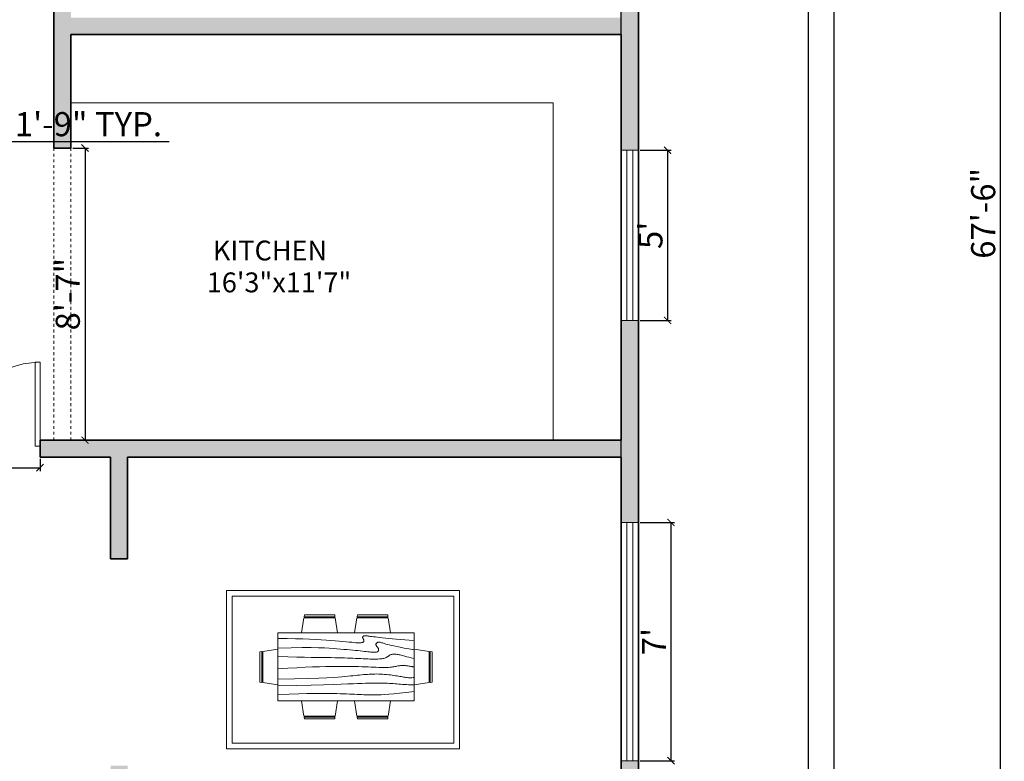
# Model space of a CAD drawing. Units: inches. Extents: x 3799 to 20199, y 1682 to 8087.
# Tile 11 of 30: x 11332 to 11679, y 2537 to 2798. Entities that reach past the tile are written whole.
import ezdxf

# ---------------------------------------------------------------- set-up
doc = ezdxf.new("R2010")
doc.units = ezdxf.units.IN
doc.linetypes.add('JIS_02_1.0', pattern=[2, 1, -1])
for name, color, linetype, lineweight in [('A-ANNO-DIMS', 2, 'Continuous', 18), ('A-AREA-IDEN', 7, 'Continuous', 18), ('A-DOOR', 3, 'Continuous', 18), ('A-FLOR-CASE', 32, 'Continuous', 18), ('A-FURN', 8, 'Continuous', 18), ('A-GLAZ', 152, 'Continuous', 18), ('A-WALL', 7, 'Continuous', 35), ('A-WALL-OVHD', 7, 'JIS_02_1.0', 18), ('A-WALL-PATT', 252, 'Continuous', 13), ('C-PROP', 7, 'Continuous', 25)]:
    doc.layers.add(name, color=color, linetype=linetype, lineweight=lineweight)
doc.styles.get("Standard").update_dxf_attribs({"font": 'arial.ttf'})
doc.dimstyles.new('ISO-25', dxfattribs={"dimtxt": 8.5, "dimasz": 2.5, "dimexe": 1.25, "dimexo": 0.625, "dimtad": 1, "dimdec": 0, "dimlunit": 3, "dimtxsty": 'Standard', "dimblk": 'ARCHTICK', "dimcen": 2.5, "dimadec": 0, "dimazin": 0, "dimtfac": 1, "dimtdec": 0, "dimtmove": 0, "dimatfit": 3, "dimfxl": 1, "dimarcsym": 0})

# ---------------------------------------------------------------- blocks, each defined once
blk = doc.blocks.new('Dining Set - 36 x 72 in.')
for p, q in [((-22, 27.5), (-22.1562, 26.50042)), ((-5.8416, 26.5), (-22.1534, 26.5)), ((-22, 27.5), (-6, 27.5)), ((-5.8437, 26.49966), (-6, 27.5)), ((6, 27.5), (5.8438, 26.50042)), ((22.1584, 26.5), (5.8466, 26.5)), ((6, 27.5), (22, 27.5)), ((22.1563, 26.49966), (22, 27.5)), ((-22.2343, 26.00059), (-23.4847, 17.99762)), ((-22.2304, 26), (-5.7608, 26)), ((-4.5152, 17.99762), (-5.7655, 25.99926)), ((5.7657, 26.00059), (4.5153, 17.99762)), ((5.7696, 26), (22.2392, 26)), ((23.4848, 17.99762), (22.2345, 25.99926)), ((36, 18), (-36, 18)), ((-36, 18), (-36, -18)), ((36, -18), (36, 18)), ((-45.5, 8), (-44.5004, 8.15617)), ((-45.5, 8), (-45.5, -8)), ((-44.5, -8.15843), (-44.5, 8.15338)), ((-44.0006, 8.23428), (-35.9976, 9.48474)), ((-44, 8.23041), (-44, -8.23915)), ((44.0006, 8.23428), (35.9976, 9.48474)), ((44, 8.23041), (44, -8.23915)), ((44.5, -8.15843), (44.5, 8.15338)), ((45.5, 8), (44.5005, 8.15617)), ((45.5, 8), (45.5, -8)), ((-44.4997, -8.15631), (-45.5, -8)), ((-35.9976, -9.48476), (-43.9993, -8.2345)), ((35.9976, -9.48476), (43.9993, -8.2345)), ((44.4997, -8.15631), (45.5, -8)), ((-36, -18), (36, -18)), ((-22.2343, -26.0006), (-23.4847, -17.99762)), ((-4.5152, -17.99762), (-5.7655, -25.99928)), ((5.7657, -26.0006), (4.5153, -17.99762)), ((23.4848, -17.99762), (22.2345, -25.99928)), ((-22.2304, -26), (-5.7608, -26)), ((5.7696, -26), (22.2392, -26)), ((-22, -27.5), (-22.1562, -26.50044)), ((-5.8416, -26.5), (-22.1534, -26.5)), ((-22, -27.5), (-6, -27.5)), ((-5.8437, -26.49967), (-6, -27.5)), ((6, -27.5), (5.8438, -26.50044)), ((22.1584, -26.5), (5.8466, -26.5)), ((6, -27.5), (22, -27.5)), ((22.1563, -26.49967), (22, -27.5))]:
    blk.add_line(p, q)
for points in [[(-36, 15), (-31.1772, 14.97754), (-26.8079, 14.91406), (-22.8538, 14.81543), (-19.276, 14.6875), (-16.0362, 14.53613), (-13.0957, 14.36718), (-10.4159, 14.18652), (-7.9583, 14), (-5.6904, 13.81315), (-3.6035, 13.63021), (-1.6954, 13.45508), (0.0365, 13.29166), (1.5945, 13.14388), (2.9811, 13.01562), (4.1988, 12.9108), (5.25, 12.83333), (6.1393, 12.78613), (6.8802, 12.76823), (7.4883, 12.77767), (7.9792, 12.8125), (8.3685, 12.87077), (8.6719, 12.95052), (8.9049, 13.0498), (9.0833, 13.16666), (9.2205, 13.29899), (9.3216, 13.44401), (9.3895, 13.59879), (9.4271, 13.76041), (9.4373, 13.92594), (9.4232, 14.09245), (9.3875, 14.257), (9.3333, 14.41666), (9.2638, 14.56917), (9.1836, 14.71484), (9.0975, 14.85465), (9.0104, 14.98958), (8.9272, 15.1206), (8.8529, 15.2487), (8.7922, 15.37483), (8.75, 15.5), (8.7305, 15.62467), (8.7344, 15.74739), (8.7617, 15.86621), (8.8125, 15.97916), (8.8867, 16.08431), (8.9844, 16.17968), (9.1055, 16.26334), (9.25, 16.33333), (9.4189, 16.38802), (9.6172, 16.42708), (9.8506, 16.45052), (10.125, 16.45833), (10.4463, 16.45052), (10.8203, 16.42708), (11.2529, 16.38802), (11.75, 16.33333), (12.3184, 16.26318), (12.9694, 16.17838), (13.7151, 16.07991), (14.5677, 15.96875), (15.5395, 15.84586), (16.6426, 15.71224), (17.8893, 15.56884), (19.2917, 15.41666), (20.859, 15.25667), (22.5879, 15.08984), (24.4721, 14.91715), (26.5052, 14.73958), (28.6809, 14.5581), (30.9929, 14.3737), (33.4347, 14.18733), (36, 14)], [(-36, 10), (-28.9766, 10.14274), (-23.1725, 10.20442), (-18.4241, 10.19775), (-14.5677, 10.13541), (-11.4399, 10.03011), (-8.877, 9.89453), (-6.7154, 9.74137), (-4.7917, 9.58333), (-2.9698, 9.43082), (-1.2246, 9.28515), (0.4415, 9.14534), (2.026, 9.01041), (3.5266, 8.87939), (4.9408, 8.7513), (6.266, 8.62516), (7.5, 8.5), (8.6411, 8.37549), (9.6914, 8.2539), (10.6538, 8.13818), (11.5312, 8.03125), (12.3267, 7.93603), (13.043, 7.85547), (13.6831, 7.79248), (14.25, 7.75), (14.7471, 7.7303), (15.1797, 7.73307), (15.5537, 7.75732), (15.875, 7.80208), (16.1494, 7.86637), (16.3828, 7.94922), (16.5811, 8.04964), (16.75, 8.16666), (16.8944, 8.29915), (17.0143, 8.44531), (17.1089, 8.60319), (17.1771, 8.77083), (17.218, 8.94629), (17.2305, 9.1276), (17.2137, 9.31282), (17.1667, 9.5), (17.0895, 9.6875), (16.987, 9.875), (16.8649, 10.0625), (16.7292, 10.25), (16.5856, 10.4375), (16.4401, 10.625), (16.2985, 10.8125), (16.1667, 11), (16.05, 11.18733), (15.9518, 11.3737), (15.8752, 11.5581), (15.8229, 11.73958), (15.798, 11.91715), (15.8034, 12.08984), (15.842, 12.25667), (15.9167, 12.41666), (16.0295, 12.56836), (16.1784, 12.70833), (16.3605, 12.83268), (16.5729, 12.9375), (16.8127, 13.01888), (17.0768, 13.07291), (17.3625, 13.0957), (17.6667, 13.08333), (17.9894, 13.03312), (18.3418, 12.94726), (18.7382, 12.82918), (19.1927, 12.68229), (19.7195, 12.51001), (20.3327, 12.31575), (21.0465, 12.10294), (21.875, 11.875), (22.8357, 11.63354), (23.959, 11.37304), (25.2786, 11.08618), (26.8282, 10.76562), (28.6414, 10.40405), (30.752, 9.99414), (33.1936, 9.52856), (36, 9)], [(-36, 5.5), (-30.7157, 5.3348), (-26.069, 5.20963), (-21.9946, 5.11767), (-18.4271, 5.05208), (-15.3009, 5.00602), (-12.5508, 4.97265), (-10.1112, 4.94515), (-7.9167, 4.91666), (-5.909, 4.88167), (-4.0586, 4.83984), (-2.3429, 4.79215), (-0.7396, 4.73958), (0.7739, 4.6831), (2.22, 4.6237), (3.6213, 4.56233), (5, 4.5), (6.373, 4.43782), (7.7344, 4.3776), (9.0723, 4.32129), (10.375, 4.27083), (11.6309, 4.22819), (12.8281, 4.19531), (13.9551, 4.17415), (15, 4.16666), (15.954, 4.17448), (16.819, 4.19791), (17.6001, 4.23698), (18.3021, 4.29166), (18.9299, 4.36198), (19.4883, 4.44791), (19.9823, 4.54948), (20.4167, 4.66666), (20.7969, 4.79899), (21.1302, 4.94401), (21.4245, 5.09879), (21.6875, 5.26041), (21.9271, 5.42594), (22.1511, 5.59245), (22.3672, 5.757), (22.5834, 5.91666), (22.8065, 6.06868), (23.0404, 6.21093), (23.2879, 6.34147), (23.5521, 6.45833), (23.8358, 6.55957), (24.142, 6.64323), (24.4735, 6.70735), (24.8334, 6.75), (25.2235, 6.76969), (25.642, 6.76692), (26.0858, 6.74267), (26.5521, 6.69791), (27.0379, 6.63362), (27.5404, 6.55078), (28.0565, 6.45036), (28.5834, 6.33333), (29.1242, 6.19987), (29.7071, 6.04687), (30.3661, 5.87044), (31.1354, 5.66666), (32.0493, 5.43164), (33.142, 5.16146), (34.4475, 4.85221), (36, 4.5)], [(-36, -1), (-30.7915, -0.6591), (-26.0195, -0.38216), (-21.6519, -0.16284), (-17.6563, 0.00521), (-14.0005, 0.12833), (-10.6523, 0.21289), (-7.5796, 0.26522), (-4.75, 0.29166), (-2.134, 0.29793), (0.2878, 0.28711), (2.5317, 0.26163), (4.6146, 0.22396), (6.5529, 0.17651), (8.3633, 0.12174), (10.0623, 0.06209), (11.6667, 0), (13.1899, -0.06201), (14.6341, -0.1211), (15.9982, -0.17432), (17.2813, -0.21875), (18.4823, -0.25147), (19.6003, -0.26953), (20.6343, -0.27002), (21.5834, -0.25), (22.4481, -0.20768), (23.2357, -0.14584), (23.9549, -0.06836), (24.6146, 0.02083), (25.2235, 0.11784), (25.7904, 0.21875), (26.3241, 0.31966), (26.8334, 0.41666), (27.3265, 0.50618), (27.8099, 0.58593), (28.2894, 0.65397), (28.7709, 0.70833), (29.2601, 0.74707), (29.763, 0.76823), (30.2855, 0.76985), (30.8334, 0.75), (31.4088, 0.70784), (31.9994, 0.64713), (32.589, 0.57275), (33.1615, 0.48958), (33.7008, 0.4025), (34.1908, 0.3164), (34.6153, 0.23616), (34.9584, 0.16666), (35.2099, 0.11165), (35.3848, 0.07031), (35.504, 0.04069), (35.5886, 0.02083), (35.6594, 0.00879), (35.7377, 0.0026), (35.8442, 0.00032), (36, 0)], [(-36, -6.5), (-27.1843, -6.31267), (-20.084, -6.1263), (-14.469, -5.9419), (-10.1094, -5.76042), (-6.7752, -5.58285), (-4.2363, -5.41016), (-2.2629, -5.24333), (-0.625, -5.08334), (0.8708, -4.93099), (2.2715, -4.78646), (3.5872, -4.64974), (4.8281, -4.52084), (6.0046, -4.39974), (7.127, -4.28646), (8.2053, -4.18099), (9.25, -4.08334), (10.2705, -3.99382), (11.2734, -3.91407), (12.2647, -3.84603), (13.25, -3.79167), (14.2354, -3.75293), (15.2266, -3.73177), (16.2295, -3.73015), (17.25, -3.75), (18.2912, -3.79248), (19.3451, -3.85547), (20.4009, -3.93604), (21.4479, -4.03125), (22.4754, -4.13819), (23.4727, -4.25391), (24.4289, -4.37549), (25.3334, -4.5), (26.1785, -4.62492), (26.9694, -4.74935), (27.7145, -4.87281), (28.4219, -4.99479), (29.1, -5.11483), (29.7572, -5.23242), (30.4016, -5.34709), (31.0417, -5.45834), (31.6837, -5.56437), (32.3262, -5.65821), (32.9658, -5.73153), (33.599, -5.77604), (34.2224, -5.78345), (34.8327, -5.74545), (35.4264, -5.65373), (36, -5.5)], [(-36, -10), (-26.4022, -9.81299), (-18.4675, -9.62891), (-11.9839, -9.45069), (-6.7396, -9.28125), (-2.5226, -9.12354), (0.8789, -8.98047), (3.6769, -8.85498), (6.0833, -8.75), (8.2767, -8.66765), (10.3021, -8.60677), (12.1712, -8.56543), (13.8958, -8.54167), (15.4876, -8.53353), (16.9583, -8.53907), (18.3197, -8.55632), (19.5834, -8.58334), (20.7616, -8.61841), (21.8685, -8.66081), (22.9188, -8.71004), (23.9271, -8.76563), (24.9081, -8.82707), (25.8763, -8.89388), (26.8465, -8.96558), (27.8334, -9.04167), (28.8474, -9.12118), (29.8828, -9.20117), (30.93, -9.27824), (31.9792, -9.34896), (33.0205, -9.40991), (34.0443, -9.45768), (35.0407, -9.48885), (36, -9.5)], [(-36, -14.5), (-30.0881, -14.33513), (-25.0332, -14.21224), (-20.7312, -14.12647), (-17.0781, -14.07292), (-13.97, -14.04671), (-11.3027, -14.04297), (-8.9724, -14.05681), (-6.875, -14.08334), (-4.9224, -14.11833), (-3.0905, -14.16016), (-1.3709, -14.20785), (0.2448, -14.26042), (1.7647, -14.3169), (3.1973, -14.3763), (4.5507, -14.43767), (5.8333, -14.5), (7.0554, -14.5621), (8.235, -14.62175), (9.3922, -14.67652), (10.5469, -14.72396), (11.7192, -14.76164), (12.929, -14.78711), (14.1965, -14.79794), (15.5417, -14.79167), (16.9933, -14.76424), (18.6152, -14.70508), (20.4804, -14.60197), (22.6615, -14.44271), (25.2312, -14.21509), (28.2624, -13.9069), (31.8277, -13.50594), (36, -13)]]:
    blk.add_lwpolyline(points)
blk = doc.blocks.new('*U47')
for p, q in [((0, 0), (0, -100)), ((750, 0), (750, -100))]:
    blk.add_line(p, q)
blk.add_lwpolyline([(0, 0), (0, 750), (43.75, 750), (43.75, 0)], close=True)
blk.add_arc((0, 0), 750, 0, 90)
blk = doc.blocks.new('_ArchTick')
at = {"color": 0, "linetype": 'ByBlock', "const_width": 0.15}
blk.add_lwpolyline([(-0.5, -0.5), (0.5, 0.5)], dxfattribs=at)
blk = doc.blocks.new('*D69')
at = {"layer": 'A-ANNO-DIMS', "color": 0, "lineweight": -2, "transparency": 16777216}
for p, q in [((11550.48, 2752.31), (11561.4, 2752.31)), ((11560.15, 2752.31), (11560.15, 2692.31)), ((11550.48, 2692.31), (11561.4, 2692.31))]:
    blk.add_line(p, q, dxfattribs=at)
at = {"layer": 'Defpoints', "color": 0, "transparency": 16777216}
for p in [(11549.85, 2752.31), (11549.85, 2692.31), (11560.15, 2692.31)]:
    blk.add_point(p, dxfattribs=at)
at = {"layer": 'A-ANNO-DIMS', "color": 0, "lineweight": -2, "transparency": 16777216, "xscale": 2.5, "yscale": 2.5, "zscale": 2.5}
for p, rotation in [((11560.15, 2752.31), 90), ((11560.15, 2692.31), 270)]:
    blk.add_blockref('_ArchTick', p, dxfattribs=dict(at, rotation=rotation))
at = {"layer": 'A-ANNO-DIMS', "color": 0, "transparency": 16777216, "insert": (11555.2, 2722.31), "char_height": 8.5, "attachment_point": 5, "rotation": 90}
blk.add_mtext("5'", dxfattribs=at)
blk = doc.blocks.new('*D70')
at = {"layer": 'A-ANNO-DIMS', "color": 0, "lineweight": -2, "transparency": 16777216}
for p, q in [((11550.48, 2621.07), (11562.6, 2621.07)), ((11561.35, 2621.07), (11561.35, 2537.07)), ((11550.48, 2537.07), (11562.6, 2537.07))]:
    blk.add_line(p, q, dxfattribs=at)
at = {"layer": 'Defpoints', "color": 0, "transparency": 16777216}
for p in [(11549.85, 2621.07), (11549.85, 2537.07), (11561.35, 2537.07)]:
    blk.add_point(p, dxfattribs=at)
at = {"layer": 'A-ANNO-DIMS', "color": 0, "lineweight": -2, "transparency": 16777216, "xscale": 2.5, "yscale": 2.5, "zscale": 2.5}
for p, rotation in [((11561.35, 2621.07), 90), ((11561.35, 2537.07), 270)]:
    blk.add_blockref('_ArchTick', p, dxfattribs=dict(at, rotation=rotation))
at = {"layer": 'A-ANNO-DIMS', "color": 0, "transparency": 16777216, "insert": (11556.48, 2579.07), "char_height": 8.5, "attachment_point": 5, "rotation": 90}
blk.add_mtext("7'", dxfattribs=at)
blk = doc.blocks.new('*D80')
at = {"layer": 'A-ANNO-DIMS', "color": 0, "lineweight": -2, "transparency": 16777216}
for p, q in [((11278.96, 2643.45), (11278.96, 2639.11)), ((11338.96, 2643.45), (11338.96, 2639.11)), ((11278.96, 2640.36), (11338.96, 2640.36))]:
    blk.add_line(p, q, dxfattribs=at)
at = {"layer": 'Defpoints', "color": 0, "transparency": 16777216}
for p in [(11278.96, 2644.07), (11338.96, 2644.07), (11338.96, 2640.36)]:
    blk.add_point(p, dxfattribs=at)
at = {"layer": 'A-ANNO-DIMS', "color": 0, "lineweight": -2, "transparency": 16777216, "xscale": 2.5, "yscale": 2.5, "zscale": 2.5, "rotation": 180}
blk.add_blockref('_ArchTick', (11278.96, 2640.36), dxfattribs=at)
at = {"layer": 'A-ANNO-DIMS', "color": 0, "lineweight": -2, "transparency": 16777216, "xscale": 2.5, "yscale": 2.5, "zscale": 2.5}
blk.add_blockref('_ArchTick', (11338.96, 2640.36), dxfattribs=at)
at = {"layer": 'A-ANNO-DIMS', "color": 0, "transparency": 16777216, "insert": (11308.96, 2645.3), "char_height": 8.5, "attachment_point": 5}
blk.add_mtext("5'", dxfattribs=at)
blk = doc.blocks.new('*D83')
at = {"layer": 'A-ANNO-DIMS', "color": 0, "lineweight": -2, "transparency": 16777216}
for p, q in [((11350.48, 2753.07), (11356.07, 2753.07)), ((11354.82, 2753.07), (11354.82, 2650.07)), ((11350.48, 2650.07), (11356.07, 2650.07))]:
    blk.add_line(p, q, dxfattribs=at)
at = {"layer": 'Defpoints', "color": 0, "transparency": 16777216}
for p in [(11349.85, 2753.07), (11349.85, 2650.07), (11354.82, 2650.07)]:
    blk.add_point(p, dxfattribs=at)
at = {"layer": 'A-ANNO-DIMS', "color": 0, "lineweight": -2, "transparency": 16777216, "xscale": 2.5, "yscale": 2.5, "zscale": 2.5}
for p, rotation in [((11354.82, 2753.07), 90), ((11354.82, 2650.07), 270)]:
    blk.add_blockref('_ArchTick', p, dxfattribs=dict(at, rotation=rotation))
at = {"layer": 'A-ANNO-DIMS', "color": 0, "transparency": 16777216, "insert": (11349.85, 2701.57), "char_height": 8.5, "attachment_point": 5, "rotation": 90}
blk.add_mtext('8\'-7"', dxfattribs=at)
blk = doc.blocks.new('WIN-60IN-6IN-FRAME')
for p, q in [((6, 60), (0, 60)), ((2, 60), (2, 0)), ((4, 60), (4, 0)), ((6, 0), (0, 0))]:
    blk.add_line(p, q)
blk = doc.blocks.new('WIN-84IN-6IN-FRAME')
for p, q in [((0, 84), (6, 84)), ((2, 0), (2, 84)), ((4, 0), (4, 84)), ((0, 0), (6, 0))]:
    blk.add_line(p, q)
blk = doc.blocks.new('*D316')
at = {"layer": 'A-ANNO-DIMS', "color": 0, "lineweight": -2, "transparency": 16777216}
for p, q in [((11267.96, 2757.88), (11267.96, 2754.13)), ((11288.8, 2757.88), (11288.8, 2754.13)), ((11267.96, 2755.38), (11288.8, 2755.38)), ((11288.8, 2755.38), (11384.5, 2755.38))]:
    blk.add_line(p, q, dxfattribs=at)
at = {"layer": 'Defpoints', "color": 0, "transparency": 16777216}
for p in [(11267.96, 2758.5), (11288.8, 2758.5), (11288.8, 2755.38)]:
    blk.add_point(p, dxfattribs=at)
at = {"layer": 'A-ANNO-DIMS', "color": 0, "lineweight": -2, "transparency": 16777216, "xscale": 2.5, "yscale": 2.5, "zscale": 2.5, "rotation": 180}
blk.add_blockref('_ArchTick', (11267.96, 2755.38), dxfattribs=at)
at = {"layer": 'A-ANNO-DIMS', "color": 0, "lineweight": -2, "transparency": 16777216, "xscale": 2.5, "yscale": 2.5, "zscale": 2.5}
blk.add_blockref('_ArchTick', (11288.8, 2755.38), dxfattribs=at)
at = {"layer": 'A-ANNO-DIMS', "color": 0, "transparency": 16777216, "insert": (11337.9, 2760.4), "char_height": 8.5, "attachment_point": 5}
blk.add_mtext('CHAIR 1\'-9" TYP.', dxfattribs=at)
blk = doc.blocks.new('*D372')
at = {"layer": 'A-ANNO-DIMS', "color": 0, "lineweight": -2, "transparency": 16777216}
for p, q in [((11543.85, 2537.7), (11543.85, 3263.92)), ((11543.85, 3262.67), (11549.85, 3262.67)), ((11549.85, 2537.7), (11549.85, 3263.92)), ((11549.85, 3262.67), (11576.2, 3262.67))]:
    blk.add_line(p, q, dxfattribs=at)
at = {"layer": 'Defpoints', "color": 0, "transparency": 16777216}
for p in [(11549.85, 3262.67), (11543.85, 2537.07), (11549.85, 2537.07)]:
    blk.add_point(p, dxfattribs=at)
at = {"layer": 'A-ANNO-DIMS', "color": 0, "lineweight": -2, "transparency": 16777216, "xscale": 2.5, "yscale": 2.5, "zscale": 2.5, "rotation": 180}
blk.add_blockref('_ArchTick', (11543.85, 3262.67), dxfattribs=at)
at = {"layer": 'A-ANNO-DIMS', "color": 0, "lineweight": -2, "transparency": 16777216, "xscale": 2.5, "yscale": 2.5, "zscale": 2.5}
blk.add_blockref('_ArchTick', (11549.85, 3262.67), dxfattribs=at)
at = {"layer": 'A-ANNO-DIMS', "color": 0, "transparency": 16777216, "insert": (11564.28, 3267.64), "char_height": 8.5, "attachment_point": 5}
blk.add_mtext('0\'-6"', dxfattribs=at)
blk = doc.blocks.new('*D374')
at = {"layer": 'A-ANNO-DIMS', "color": 0, "lineweight": -2, "transparency": 16777216}
for p, q in [((11550.48, 3135.07), (11678.7, 3135.07)), ((11677.45, 2325.07), (11677.45, 3135.07)), ((11550.48, 2325.07), (11678.7, 2325.07))]:
    blk.add_line(p, q, dxfattribs=at)
at = {"layer": 'Defpoints', "color": 0, "transparency": 16777216}
for p in [(11549.85, 3135.07), (11677.45, 3135.07), (11549.85, 2325.07)]:
    blk.add_point(p, dxfattribs=at)
at = {"layer": 'A-ANNO-DIMS', "color": 0, "lineweight": -2, "transparency": 16777216, "xscale": 2.5, "yscale": 2.5, "zscale": 2.5}
for p, rotation in [((11677.45, 3135.07), 90), ((11677.45, 2325.07), 270)]:
    blk.add_blockref('_ArchTick', p, dxfattribs=dict(at, rotation=rotation))
at = {"layer": 'A-ANNO-DIMS', "color": 0, "transparency": 16777216, "insert": (11672.49, 2730.07), "char_height": 8.5, "attachment_point": 5, "rotation": 90}
blk.add_mtext('67\'-6"', dxfattribs=at)

msp = doc.modelspace()

# ---------------------------------------------------------------- hatches: boundary and pattern name
at = {"layer": 'A-WALL-PATT'}
h = msp.add_hatch(color=256, dxfattribs=at)
h.dxf.hatch_style = 1
h.paths.add_polyline_path([(11549.85, 2537.07), (11543.85, 2537.07), (11543.85, 2493.07), (11500.92, 2493.07), (11500.92, 2487.07), (11543.85, 2487.07), (11543.85, 2331.07), (11512.59, 2331.07), (11512.59, 2325.07), (11549.85, 2325.07)])
h.paths.add_polyline_path([(11404.92, 2493.07), (11369.85, 2493.07), (11369.85, 2535.29), (11363.85, 2535.29), (11363.85, 2493.07), (11359.67, 2493.07), (11359.67, 2487.07), (11404.92, 2487.07)])
h.paths.add_polyline_path([(11347.67, 2493.07), (11315.85, 2493.07), (11315.85, 2481.32), (11321.85, 2481.32), (11321.85, 2487.07), (11347.67, 2487.07)])
h.paths.add_polyline_path([(11246.96, 2394.07), (11231.85, 2394.07), (11231.85, 2493.07), (11126.81, 2493.07), (11126.81, 2487.07), (11225.85, 2487.07), (11225.85, 2325.07), (11315.85, 2325.07), (11315.85, 2331.07), (11231.85, 2331.07), (11231.85, 2388.07), (11246.96, 2388.07)])
h.paths.add_polyline_path([(11368.59, 2331.07), (11321.85, 2331.07), (11321.85, 2421.32), (11319.79, 2421.32), (11315.85, 2421.32), (11315.85, 2394.07), (11306.96, 2394.07), (11306.96, 2392.01), (11306.96, 2388.07), (11315.85, 2388.07), (11315.85, 2325.07), (11368.59, 2325.07)])
h.paths.add_polyline_path([(11211.5, 2599.62), (11175.25, 2599.62), (11175.25, 2594.62), (11206.5, 2594.62), (11206.5, 2541.62), (11137.5, 2541.62), (11137.5, 2594.62), (11145.25, 2594.62), (11145.25, 2599.62), (11132.5, 2599.62), (11132.5, 2536.62), (11211.5, 2536.62)], flags=17)
h.paths.add_polyline_path([(11278.96, 2650.07), (11117.85, 2650.07), (11117.85, 2668.07), (11111.85, 2668.07), (11111.85, 2650.07), (11087.85, 2650.07), (11087.85, 2526.57), (11093.85, 2526.57), (11093.85, 2644.07), (11278.96, 2644.07)])
h.paths.add_polyline_path([(11096.81, 2491.01), (11096.81, 2493.07), (11093.85, 2493.07), (11093.85, 2496.57), (11087.85, 2496.57), (11087.85, 2487.07), (11096.81, 2487.07)])
h.paths.add_polyline_path([(11445.85, 3087.71), (11439.85, 3087.71), (11439.85, 2949.07), (11343.85, 2949.07), (11343.85, 2929.61), (11315.6, 2929.61), (11315.6, 2923.61), (11343.85, 2923.61), (11343.85, 2840.12), (11349.85, 2840.12), (11349.85, 2943.07), (11507.11, 2943.07), (11507.11, 2949.07), (11445.85, 2949.07), (11445.85, 3015.07), (11543.85, 3015.07), (11543.85, 2992.92), (11549.85, 2992.92), (11549.85, 3108.28), (11543.85, 3108.28), (11543.85, 3021.07), (11515.89, 3021.07), (11515.89, 3049.36), (11511.89, 3049.36), (11511.89, 3021.07), (11445.85, 3021.07)])
h.paths.add_polyline_path([(11549.85, 3135.07), (11408.12, 3135.07), (11408.12, 3129.07), (11439.85, 3129.07), (11439.85, 3117.71), (11443.79, 3117.71), (11445.85, 3117.71), (11445.85, 3129.07), (11504.47, 3129.07), (11504.47, 3099.65), (11508.47, 3099.65), (11508.47, 3129.07), (11543.85, 3129.07), (11543.85, 3126.28), (11549.85, 3126.28)])
h.paths.add_polyline_path([(11324.12, 3135.07), (11087.85, 3135.07), (11087.85, 3083.46), (11093.85, 3083.46), (11093.85, 3129.07), (11265.85, 3129.07), (11265.85, 3050.07), (11240.75, 3050.07), (11240.75, 3044.07), (11265.85, 3044.07), (11265.85, 2895.64), (11271.85, 2895.64), (11271.85, 2923.61), (11279.6, 2923.61), (11279.6, 2929.61), (11271.85, 2929.61), (11271.85, 3129.07), (11324.12, 3129.07)])
h.paths.add_polyline_path([(11210.75, 3050.07), (11133.85, 3050.07), (11133.85, 3088.63), (11129.85, 3088.54), (11129.85, 3050.07), (11093.85, 3050.07), (11093.85, 3059.46), (11087.85, 3059.46), (11087.85, 3030.25), (11093.85, 3030.25), (11093.85, 3044.07), (11210.75, 3044.07)], flags=17)
h.paths.add_polyline_path([(11093.85, 2982.25), (11087.85, 2982.25), (11087.85, 2913.95), (11093.85, 2913.95)], flags=17)
h.paths.add_polyline_path([(11271.85, 2859.64), (11265.85, 2859.64), (11265.85, 2854.07), (11093.85, 2854.07), (11093.85, 2865.95), (11087.85, 2865.95), (11087.85, 2848.07), (11111.85, 2848.07), (11111.85, 2812.07), (11117.85, 2812.07), (11117.85, 2848.07), (11271.85, 2848.07)])
h.paths.add_polyline_path([(11549.85, 2847.23), (11543.85, 2847.23), (11543.85, 2799.07), (11349.85, 2799.07), (11349.85, 2804.12), (11343.85, 2804.12), (11343.85, 2753.07), (11349.85, 2753.07), (11349.85, 2793.07), (11543.85, 2793.07), (11543.85, 2752.31), (11549.85, 2752.31)])
h.paths.add_polyline_path([(11549.85, 2692.31), (11543.85, 2692.31), (11543.85, 2650.07), (11343.85, 2650.07), (11338.96, 2650.07), (11338.96, 2644.07), (11349.85, 2644.07), (11363.85, 2644.07), (11363.85, 2608.29), (11369.85, 2608.29), (11369.85, 2644.07), (11543.85, 2644.07), (11543.85, 2621.07), (11549.85, 2621.07)])

# ---------------------------------------------------------------- linework, layer by layer
at = {"layer": 'A-FLOR-CASE'}
for p, q in [((11519.85, 2769.07), (11349.85, 2769.07)), ((11519.85, 2650.07), (11519.85, 2769.07))]:
    msp.add_line(p, q, dxfattribs=at)
at = {"layer": 'A-FURN'}
for points in [[(11404.71, 2597.03), (11486.86, 2597.03), (11486.86, 2541.2), (11404.71, 2541.2)], [(11406.71, 2595.03), (11484.86, 2595.03), (11484.86, 2543.2), (11406.71, 2543.2)]]:
    msp.add_lwpolyline(points, close=True, dxfattribs=at)
at = {"layer": 'A-WALL'}
for p, q in [((11549.85, 2325.07), (11549.85, 3135.07)), ((11343.85, 2753.07), (11343.85, 2804.12)), ((11543.85, 2793.07), (11349.85, 2793.07)), ((11349.85, 2753.07), (11349.85, 2793.07)), ((11543.85, 2650.07), (11543.85, 2793.07)), ((11343.85, 2753.07), (11349.85, 2753.07)), ((11343.85, 2650.07), (11338.96, 2650.07)), ((11338.96, 2650.07), (11338.96, 2644.07)), ((11343.85, 2650.07), (11543.85, 2650.07)), ((11349.85, 2644.07), (11338.96, 2644.07)), ((11349.85, 2644.07), (11363.85, 2644.07)), ((11363.85, 2608.29), (11363.85, 2644.07)), ((11369.85, 2644.07), (11543.85, 2644.07)), ((11369.85, 2608.29), (11369.85, 2644.07)), ((11543.85, 2493.07), (11543.85, 2644.07)), ((11363.85, 2608.29), (11369.85, 2608.29))]:
    msp.add_line(p, q, dxfattribs=at)
at = {"layer": 'A-WALL-OVHD'}
for p, q in [((11343.85, 2753.07), (11343.85, 2650.07)), ((11349.85, 2753.07), (11349.85, 2650.07))]:
    msp.add_line(p, q, dxfattribs=at)
at = {"layer": 'C-PROP'}
for p, q in [((11618.85, 2124.07), (11618.85, 3204.07)), ((11609.85, 2133.07), (11609.85, 3195.07))]:
    msp.add_line(p, q, dxfattribs=at)

# ---------------------------------------------------------------- block references
at = {"layer": 'A-DOOR', "xscale": -0.0393700787401575, "yscale": 0.0393700787401575, "zscale": 0.0393700787401575}
msp.add_blockref('*U47', (11338.96, 2648.01), dxfattribs=at)
at = {"layer": 'A-FURN', "xscale": 0.6667335619926691, "yscale": 0.6667335619926691, "zscale": 0.6667335619926691}
msp.add_blockref('Dining Set - 36 x 72 in.', (11446.83, 2570.12), dxfattribs=at)
at = {"layer": 'A-GLAZ'}
for name, p in [('WIN-60IN-6IN-FRAME', (11543.85, 2692.31)), ('WIN-84IN-6IN-FRAME', (11543.85, 2537.07))]:
    msp.add_blockref(name, p, dxfattribs=at)

# ---------------------------------------------------------------- texts
at = {"layer": 'A-AREA-IDEN'}
for s, p in [(' KITCHEN', (11397.75, 2713.45)), ('16\'3"x11\'7"', (11397.75, 2702.21))]:
    msp.add_text(s, height=7, rotation=0.0019, dxfattribs=at).set_placement(p)

# ---------------------------------------------------------------- dimensions: what is measured, and where the dimension line sits
at = {"layer": 'A-ANNO-DIMS'}
for base, p1, p2, override, picture, middle in [((11549.85, 3262.67), (11543.85, 2537.07), (11549.85, 2537.07), {"dimdec": 1, "dimlfac": 1, "dimrnd": 0, "dimzin": 1, "dimdsep": 46, "dimlunit": 4, "dimfrac": 2}, '*D372', (11564.28, 3267.64)), ((11338.96, 2640.36), (11278.96, 2644.07), (11338.96, 2644.07), {"dimclrd": 0, "dimclre": 0, "dimclrt": 0}, '*D80', (11308.96, 2645.3))]:
    dim = msp.add_linear_dim(base=base, p1=p1, p2=p2, dimstyle='ISO-25', override=override, dxfattribs=at)
    dim.commit()
    dim.dimension.update_dxf_attribs({"geometry": picture, "text_midpoint": middle})
for base, p1, p2, override, picture, middle in [((11677.45, 3135.07), (11549.85, 2325.07), (11549.85, 3135.07), {"dimdec": 1, "dimlfac": 1, "dimrnd": 0, "dimzin": 1, "dimdsep": 46, "dimlunit": 4, "dimfrac": 2}, '*D374', (11672.49, 2730.07)), ((11354.82, 2650.07), (11349.85, 2753.07), (11349.85, 2650.07), {"dimclrd": 0, "dimclre": 0, "dimclrt": 0}, '*D83', (11349.85, 2701.57)), ((11560.15, 2692.31), (11549.85, 2752.31), (11549.85, 2692.31), {"dimclrd": 0, "dimclre": 0, "dimclrt": 0}, '*D69', (11555.2, 2722.31)), ((11561.35, 2537.07), (11549.85, 2621.07), (11549.85, 2537.07), {"dimclrd": 0, "dimclre": 0, "dimclrt": 0}, '*D70', (11556.48, 2579.07))]:
    dim = msp.add_linear_dim(base=base, p1=p1, p2=p2, angle=90, dimstyle='ISO-25', override=override, dxfattribs=at)
    dim.commit()
    dim.dimension.update_dxf_attribs({"geometry": picture, "text_midpoint": middle})
dim = msp.add_linear_dim(base=(11288.8, 2755.38), p1=(11267.96, 2758.5), p2=(11288.8, 2758.5), angle=0, text='CHAIR <> TYP.', dimstyle='ISO-25', override={"dimdec": 1, "dimlfac": 1, "dimrnd": 0, "dimzin": 1, "dimdsep": 46, "dimlunit": 4, "dimfrac": 2}, dxfattribs=at)
dim.commit()
dim.dimension.update_dxf_attribs({"geometry": '*D316', "text_midpoint": (11337.9, 2760.4)})

doc.saveas('drawing.dxf')
